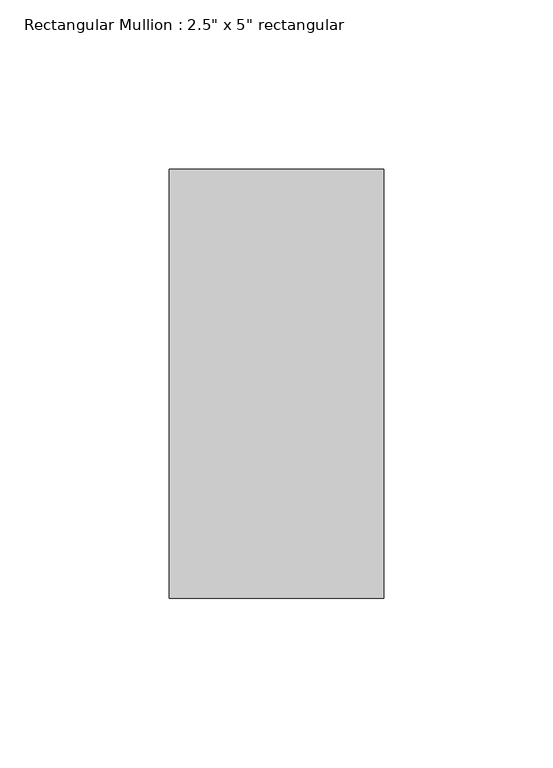
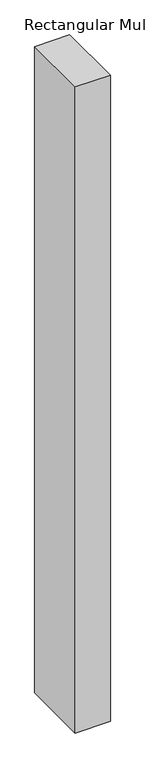
"""IFC4 building model written with IfcOpenShell, lengths in millimetres: member geometry."""

from ifc_helpers import new_model, si_unit, frame, origin, place, context, project, spatial, polyline, outline, extrude, source, transform, mapped, element, save


def member_2caf7d25(model_context):
    return source(origin(), model_context, "Body", "SweptSolid", [
        extrude(outline(polyline([(0.0, 63.5), (0.0, -63.5), (-63.5, -63.5), (-63.5, 63.5), (0.0, 63.5)])), frame((0.0, 0.0, -1236.7434076), z_axis=(0.0, 0.0, 1.0), x_axis=(1.0, 0.0, 0.0)), (0.0, 0.0, 1.0), 1236.7434076),
    ])


if __name__ == "__main__":
    model = new_model("IFC4")
    model_context = context("Model", 3, world=origin())
    ifc_project = project(units=[si_unit("LENGTHUNIT", "METRE", prefix="MILLI")], contexts=[model_context])
    site = spatial("IfcSite", under=ifc_project)
    building = spatial("IfcBuilding", under=site)
    placement = place(None, origin())
    member_shape = member_2caf7d25(model_context)
    element("IfcMember", 1, ObjectType="Rectangular Mullion : 2.5\" x 5\" rectangular", at=placement, inside=building, context=model_context, shape_type="MappedRepresentation", body=[
        mapped(member_shape, transform((0.0, 0.0, 0.0), x_axis=(1.0, 0.0, 0.0), y_axis=(0.0, 1.0, 0.0), z_axis=(0.0, 0.0, 1.0))),
    ])
    save(model, "model.ifc")

# Revit data of these elements
# Type "Rectangular Mullion : 2.5\" x 5\" rectangular"
#   built-in parameter 1007304 = 0.416667 (stored number, unit not read)
#   built-in parameter 1007301 = 0.104167 (stored number, unit not read)
#   built-in parameter 1007300 = 0.104167 (stored number, unit not read)
# Element 1 (IfcMember, "Rectangular Mullion : 2.5\" x 5\" rectangular")
#   Materials on its faces: "Aluminum"
# Materials
#   "Aluminum": class "Metal", colour RGB 247 247 247, transparency 0, Description = "Aluminum 6061", Cost = 0
